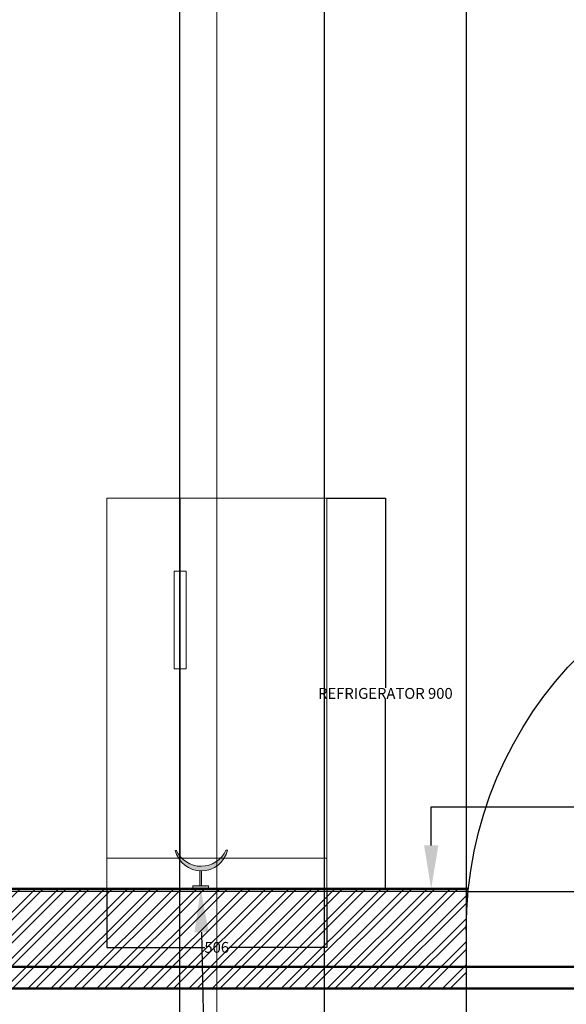
# Model space of a CAD drawing. Units: millimetres. Extents: x 1944 to 29915, y -10550 to 5909.
# Tile 5 of 24: x 7967 to 9226, y -5 to 2263. Entities that reach past the tile are written whole.
import ezdxf
from ezdxf import colors
from ezdxf.entities.mleader import LeaderData, LeaderLine
from ezdxf.math import Vec2, Vec3

# ---------------------------------------------------------------- set-up
doc = ezdxf.new("R2010")
doc.units = ezdxf.units.MM
doc.header["$MEASUREMENT"] = 0
for name, color, linetype, lineweight in [('A-ANNO-DIMS', 2, 'Continuous', 18), ('A-ANNO-SYMB', 2, 'Continuous', 18), ('A-ANNO-TEXT', 7, 'Continuous', 25), ('A-DOOR', 4, 'Continuous', 25), ('A-FLOR-FIXT', 9, 'Continuous', 18), ('A-FURN', 8, 'Continuous', 18), ('A-WALL', 7, 'Continuous', 50), ('A-WALL-PATT', 8, 'Continuous', 18)]:
    doc.layers.add(name, color=color, linetype=linetype, lineweight=lineweight)
doc.styles.get("Standard").update_dxf_attribs({"font": 'arial.ttf'})
doc.dimstyles.get("Standard").update_dxf_attribs({"dimtxt": 25, "dimasz": 0.18, "dimexe": 0.18, "dimexo": 0.0625, "dimgap": 0.09, "dimtad": 0, "dimtih": 1, "dimtoh": 1, "dimdec": 0, "dimzin": 0, "dimdsep": 46, "dimtxsty": 'Standard', "dimcen": 0.09, "dimadec": 0, "dimazin": 0, "dimtfac": 1, "dimtdec": 0, "dimtofl": 0, "dimtmove": 0, "dimatfit": 3, "dimfxl": 1, "dimtolj": 1, "dimtzin": 0, "dimarcsym": 0})

# ---------------------------------------------------------------- blocks, each defined once
blk = doc.blocks.new('*U2')
for p, q in [((0, 0), (0, -6)), ((40, 0), (40, -6))]:
    blk.add_line(p, q)
blk.add_lwpolyline([(0, 0), (0, 40), (1.75, 40), (1.75, 0)], close=True)
blk.add_arc((0, 0), 40, 0, 90)
blk = doc.blocks.new('Refrigerator-2 door - 36 in front')
for p, q in [((12, 5), (12, 64)), ((0, 5), (36, 5))]:
    blk.add_line(p, q)
for points in [[(0, 0), (0, 64), (36, 64), (36, 0)], [(11, 36), (11, 52), (13, 52), (13, 36)]]:
    blk.add_lwpolyline(points, close=True)
blk = doc.blocks.new('COAT-HOOK')
blk.add_line((47.6, 3.3), (47.6, 0))
for centre, radius, start, end in [((61.9, 60.2), 61.9, 103.3534, 256.6466), ((73.3, 60.6), 62.7, 114.1736, 245.8264)]:
    blk.add_arc(centre, radius, start, end)
blk = doc.blocks.new('*D40')
at = {"layer": 'A-ANNO-DIMS', "color": 0, "lineweight": -2, "transparency": 16777216}
for p, q in [((8674.1, 1160.8), (8809.2, 1160.8)), ((8809.1, 1160.7), (8809.1, 723.9)), ((8809.1, 261), (8809.1, 697.8)), ((8674.1, 260.8), (8809.2, 260.8))]:
    blk.add_line(p, q, dxfattribs=at)
at = {"layer": 'A-ANNO-DIMS', "color": 0, "transparency": 16777216}
for points in [[(8809, 1160.7), (8809.1, 1160.7), (8809.1, 1160.8)], [(8809, 261), (8809.1, 261), (8809.1, 260.8)]]:
    blk.add_solid(points, dxfattribs=at)
at = {"layer": 'Defpoints', "color": 0, "transparency": 16777216}
for p in [(8674.1, 1160.8), (8809.1, 1160.8), (8674.1, 260.8)]:
    blk.add_point(p, dxfattribs=at)
at = {"layer": 'A-ANNO-DIMS', "color": 0, "transparency": 16777216, "insert": (8809.1, 710.8), "char_height": 25, "attachment_point": 5}
blk.add_mtext('\\A1;REFRIGERATOR 900', dxfattribs=at)
blk = doc.blocks.new('*D41')
at = {"layer": 'A-ANNO-DIMS', "color": 0, "lineweight": -2, "transparency": 16777216}
for p, q in [((8167.8, 260.8), (8167.8, 125.7)), ((8674.1, 260.8), (8674.1, 125.7)), ((8168, 125.8), (8393.2, 125.8)), ((8673.9, 125.8), (8448.6, 125.8))]:
    blk.add_line(p, q, dxfattribs=at)
at = {"layer": 'A-ANNO-DIMS', "color": 0, "transparency": 16777216}
for points in [[(8168, 125.9), (8168, 125.8), (8167.8, 125.8)], [(8673.9, 125.9), (8673.9, 125.8), (8674.1, 125.8)]]:
    blk.add_solid(points, dxfattribs=at)
at = {"layer": 'Defpoints', "color": 0, "transparency": 16777216}
for p in [(8167.8, 260.8), (8674.1, 260.8), (8674.1, 125.8)]:
    blk.add_point(p, dxfattribs=at)
at = {"layer": 'A-ANNO-DIMS', "color": 0, "transparency": 16777216, "insert": (8420.9, 125.8), "char_height": 25, "attachment_point": 5}
blk.add_mtext('\\A1;506', dxfattribs=at)
blk = doc.blocks.new('*D49')
at = {"layer": 'A-ANNO-DIMS', "color": 0, "lineweight": -2, "transparency": 16777216}
for p, q in [((8335.5, 4760.8), (8335.5, -697.2)), ((6945.9, 4530.8), (6945.9, -697.2)), ((6946.1, -697), (7589.8, -697)), ((8335.3, -697), (7691.6, -697))]:
    blk.add_line(p, q, dxfattribs=at)
at = {"layer": 'A-ANNO-DIMS', "color": 0, "transparency": 16777216}
for points in [[(6946.1, -697), (6946.1, -697.1), (6945.9, -697)], [(8335.3, -697), (8335.3, -697.1), (8335.5, -697)]]:
    blk.add_solid(points, dxfattribs=at)
at = {"layer": 'Defpoints', "color": 0, "transparency": 16777216}
for p in [(8335.5, 4760.8), (6945.9, 4530.8), (8335.5, -697)]:
    blk.add_point(p, dxfattribs=at)
at = {"layer": 'A-ANNO-DIMS', "color": 0, "transparency": 16777216, "insert": (7640.7, -697), "char_height": 25, "attachment_point": 5}
blk.add_mtext('\\A1;1389.5', dxfattribs=at)
blk = doc.blocks.new('*D50')
at = {"layer": 'A-ANNO-DIMS', "color": 0, "lineweight": -2, "transparency": 16777216}
for p, q in [((8995.2, 30.8), (8995.2, -697.2)), ((9895.2, 30.8), (9895.2, -697.2)), ((8995.4, -697), (9417.6, -697)), ((9895, -697), (9472.9, -697))]:
    blk.add_line(p, q, dxfattribs=at)
at = {"layer": 'A-ANNO-DIMS', "color": 0, "transparency": 16777216}
for points in [[(8995.4, -697), (8995.4, -697.1), (8995.2, -697)], [(9895, -697), (9895, -697.1), (9895.2, -697)]]:
    blk.add_solid(points, dxfattribs=at)
at = {"layer": 'Defpoints', "color": 0, "transparency": 16777216}
for p in [(8995.2, 30.8), (9895.2, 30.8), (9895.2, -697)]:
    blk.add_point(p, dxfattribs=at)
at = {"layer": 'A-ANNO-DIMS', "color": 0, "transparency": 16777216, "insert": (9445.2, -697), "char_height": 25, "attachment_point": 5}
blk.add_mtext('\\A1;900', dxfattribs=at)
blk = doc.blocks.new('*D53')
at = {"layer": 'A-ANNO-DIMS', "color": 0, "lineweight": -2, "transparency": 16777216}
for p, q in [((6945.94205, 490.774608), (6945.94205, -697.212556)), ((9895.94205, 490.774608), (9895.94205, -697.212556)), ((6946.12205, -697.032556), (8383.35205, -697.032556)), ((9895.76205, -697.032556), (8458.53205, -697.032556))]:
    blk.add_line(p, q, dxfattribs=at)
at = {"layer": 'A-ANNO-DIMS', "color": 0, "transparency": 16777216}
for points in [[(6946.12205, -697.002556), (6946.12205, -697.062556), (6945.94205, -697.032556)], [(9895.76205, -697.002556), (9895.76205, -697.062556), (9895.94205, -697.032556)]]:
    blk.add_solid(points, dxfattribs=at)
at = {"layer": 'Defpoints', "color": 0, "transparency": 16777216}
for p in [(6945.94205, 490.837108), (9895.94205, 490.837108), (9895.94205, -697.032556)]:
    blk.add_point(p, dxfattribs=at)
at = {"layer": 'A-ANNO-DIMS', "color": 0, "transparency": 16777216, "insert": (8420.94205, -697.032556), "char_height": 25, "attachment_point": 5}
blk.add_mtext('\\A1;2950', dxfattribs=at)
blk = doc.blocks.new('*D56')
at = {"layer": 'A-ANNO-DIMS', "color": 0, "lineweight": -2, "transparency": 16777216}
for p, q in [((8999.7, 254.8), (11007.7, 254.8)), ((11007.5, 254.6), (11007.5, 155.7)), ((11007.5, 31), (11007.5, 130)), ((8995.3, 30.8), (11007.7, 30.8))]:
    blk.add_line(p, q, dxfattribs=at)
at = {"layer": 'A-ANNO-DIMS', "color": 0, "transparency": 16777216}
for points in [[(11007.5, 254.6), (11007.5, 254.6), (11007.5, 254.8)], [(11007.5, 31), (11007.5, 31), (11007.5, 30.8)]]:
    blk.add_solid(points, dxfattribs=at)
at = {"layer": 'Defpoints', "color": 0, "transparency": 16777216}
for p in [(8999.6, 254.8), (8995.2, 30.8), (11007.5, 30.8)]:
    blk.add_point(p, dxfattribs=at)
at = {"layer": 'A-ANNO-DIMS', "color": 0, "transparency": 16777216, "insert": (11007.5, 142.8), "char_height": 25, "attachment_point": 5}
blk.add_mtext('\\A1;223.95', dxfattribs=at)
blk = doc.blocks.new('*D57')
at = {"layer": 'A-ANNO-DIMS', "color": 0, "lineweight": -2, "transparency": 16777216}
for p, q in [((8995.2, 4760.8), (5803.8, 4760.8)), ((5804, 4760.7), (5804, 2520.7)), ((5804, 255), (5804, 2495)), ((8999.6, 254.8), (5803.8, 254.8))]:
    blk.add_line(p, q, dxfattribs=at)
at = {"layer": 'A-ANNO-DIMS', "color": 0, "transparency": 16777216}
for points in [[(5804, 4760.7), (5804, 4760.7), (5804, 4760.8)], [(5804, 255), (5804, 255), (5804, 254.8)]]:
    blk.add_solid(points, dxfattribs=at)
at = {"layer": 'Defpoints', "color": 0, "transparency": 16777216}
for p in [(8995.2, 4760.8), (5804, 254.8), (8999.6, 254.8)]:
    blk.add_point(p, dxfattribs=at)
at = {"layer": 'A-ANNO-DIMS', "color": 0, "transparency": 16777216, "insert": (5804, 2507.8), "char_height": 25, "attachment_point": 5}
blk.add_mtext('\\A1;4506', dxfattribs=at)
blk = doc.blocks.new('*D59')
at = {"layer": 'A-ANNO-DIMS', "color": 0, "lineweight": -2, "transparency": 16777216}
for p, q in [((8668, 4019.6), (8668, -697.2)), ((8995.2, 3870.8), (8995.2, -697.2)), ((8668.2, -697), (8789.5, -697)), ((8995, -697), (8873.8, -697))]:
    blk.add_line(p, q, dxfattribs=at)
at = {"layer": 'A-ANNO-DIMS', "color": 0, "transparency": 16777216}
for points in [[(8668.2, -697), (8668.2, -697.1), (8668, -697)], [(8995, -697), (8995, -697.1), (8995.2, -697)]]:
    blk.add_solid(points, dxfattribs=at)
at = {"layer": 'Defpoints', "color": 0, "transparency": 16777216}
for p in [(8668, 4019.6), (8995.2, 3870.8), (8995.2, -697)]:
    blk.add_point(p, dxfattribs=at)
at = {"layer": 'A-ANNO-DIMS', "color": 0, "transparency": 16777216, "insert": (8831.6, -697), "char_height": 25, "attachment_point": 5}
blk.add_mtext('\\A1;327.2', dxfattribs=at)

msp = doc.modelspace()

# ---------------------------------------------------------------- hatches: boundary and pattern name
at = {"layer": 'A-ANNO-SYMB'}
h = msp.add_hatch(color=256, dxfattribs=at)
h.dxf.hatch_style = 1
h.paths.add_polyline_path([(8445.574, 349.638), (8442.267, 349.638, -0.64725624), (8327.774, 349.638), (8325.088, 349.638, 0.79041326)])
h = msp.add_hatch(color=256, dxfattribs=at)
h.dxf.hatch_style = 1
h.paths.add_polyline_path([(8382.09, 267.383), (8386.174, 267.383), (8386.174, 302.026, -0.01650068), (8382.09, 302.106)])
h = msp.add_hatch(color=256, dxfattribs=at)
h.dxf.hatch_style = 1
h.paths.add_polyline_path([(8402.167, 260.837), (8402.167, 267.383), (8365.937, 267.383), (8365.937, 260.837)])
at = {"layer": 'A-WALL-PATT'}
h = msp.add_hatch(dxfattribs=at)
h.set_pattern_fill('ANSI32', color=256, scale=100)
h.paths.add_polyline_path([(6945.942, 260.837), (6945.942, 30.837), (8995.217, 30.837), (8995.217, 165.837, -0.0264443), (9000.245, 260.837)])

# ---------------------------------------------------------------- linework, layer by layer
at = {"layer": 'A-ANNO-SYMB'}
msp.add_line((8420.942, -176.269), (8420.942, 5412.489), dxfattribs=at)
at = {"layer": 'A-FLOR-FIXT'}
for p, q in [((8382.09, 302.089), (8382.09, 267.383)), ((8386.174, 302.089), (8386.174, 267.383))]:
    msp.add_line(p, q, dxfattribs=at)
for points in [[(8995.217, 30.837), (6715.942, 30.837), (6715.942, 4990.837), (8315.477, 4990.837)], [(9000.245, 260.837), (6945.942, 260.837), (6945.942, 4760.837), (8315.477, 4760.837)]]:
    msp.add_lwpolyline(points, dxfattribs=at)
msp.add_lwpolyline([(8402.167, 260.837), (8365.937, 260.837), (8365.937, 267.383), (8402.167, 267.383)], close=True, dxfattribs=at)
at = {"layer": 'A-WALL'}
for p, q in [((6945.942, 260.837), (9000.245, 260.837)), ((10125.942, 81.017), (6715.942, 81.017)), ((10125.942, 30.837), (6715.942, 30.837)), ((8995.217, 30.837), (9895.942, 30.837))]:
    msp.add_line(p, q, dxfattribs=at)

# ---------------------------------------------------------------- block references
at = {"layer": 'A-DOOR', "xscale": -22.5, "yscale": 22.5, "zscale": 22.5}
msp.add_blockref('*U2', (9895.217, 165.837), dxfattribs=at)
at = {"layer": 'A-FLOR-FIXT', "xscale": 14.0625, "yscale": 14.0625, "zscale": 14.0625}
msp.add_blockref('Refrigerator-2 door - 36 in front', (8167.817, 260.837), dxfattribs=at)
at = {"layer": 'A-FURN', "rotation": 90.14209801514701}
msp.add_blockref('COAT-HOOK', (8445.704, 302.134), dxfattribs=at)

# ---------------------------------------------------------------- dimensions: what is measured, and where the dimension line sits
at = {"layer": 'A-ANNO-DIMS'}
for base, p1, p2, override, picture, middle in [((5803.984, 254.791), (8995.217, 4760.837), (8999.621, 254.791), {"dimdec": 0, "dimlfac": 1, "dimrnd": 0, "dimzin": 0, "dimdsep": 46, "dimlunit": 2}, '*D57', (5803.984, 2507.814)), ((11007.504, 30.837), (8999.621, 254.791), (8995.217, 30.837), {"dimdec": 2, "dimlfac": 1, "dimrnd": 0, "dimzin": 0, "dimdsep": 46, "dimlunit": 2}, '*D56', (11007.504, 142.814))]:
    dim = msp.add_linear_dim(base=base, p1=p1, p2=p2, angle=90, dimstyle='Standard', override=override, dxfattribs=at)
    dim.commit()
    dim.dimension.update_dxf_attribs({"geometry": picture, "text_midpoint": middle})
for base, p1, p2, override, picture, middle in [((8335.477, -697.033), (6945.942, 4530.837), (8335.477, 4760.837), {"dimdec": 1, "dimlfac": 1, "dimrnd": 0, "dimzin": 0, "dimdsep": 46, "dimlunit": 2}, '*D49', (7640.71, -697.033)), ((8995.217, -697.033), (8668.038, 4019.643), (8995.217, 3870.837), {"dimdec": 1, "dimlfac": 1, "dimrnd": 0, "dimzin": 0, "dimdsep": 46, "dimlunit": 2}, '*D59', (8831.628, -697.033)), ((9895.942, -697.033), (6945.942, 490.837), (9895.942, 490.837), {"dimdec": 0, "dimlfac": 1, "dimrnd": 0, "dimzin": 0, "dimdsep": 46, "dimlunit": 2}, '*D53', (8420.942, -697.033)), ((8674.067, 125.837), (8167.817, 260.837), (8674.067, 260.837), {"dimdec": 0, "dimrnd": 0, "dimzin": 0, "dimlunit": 2}, '*D41', (8420.942, 125.837)), ((9895.217, -697.033), (8995.217, 30.837), (9895.217, 30.837), {"dimdec": 0, "dimlfac": 1, "dimrnd": 0, "dimzin": 0, "dimdsep": 46, "dimlunit": 2}, '*D50', (9445.217, -697.033))]:
    dim = msp.add_linear_dim(base=base, p1=p1, p2=p2, dimstyle='Standard', override=override, dxfattribs=at)
    dim.commit()
    dim.dimension.update_dxf_attribs({"geometry": picture, "text_midpoint": middle})
dim = msp.add_linear_dim(base=(8809.067, 1160.837), p1=(8674.067, 260.837), p2=(8674.067, 1160.837), angle=90, text='REFRIGERATOR <>', dimstyle='Standard', override={"dimdec": 0, "dimrnd": 0, "dimzin": 0, "dimlunit": 2}, dxfattribs=at)
dim.commit()
dim.dimension.update_dxf_attribs({"geometry": '*D40', "text_midpoint": (8809.067, 710.837)})

# ---------------------------------------------------------------- leaders
at = {"layer": 'A-ANNO-TEXT'}
ml = msp.add_multileader_mtext('Standard', dxfattribs=at)
ml.set_content('SWITCH BOARD', color=256)
ml.set_leader_properties()
ml.build(insert=Vec2(0, 0))
ml.multileader.update_dxf_attribs({"dogleg_length": 568.936, "arrow_head_size": 100})
ctx = ml.context
ctx.base_point, ctx.char_height, ctx.arrow_head_size, ctx.landing_gap_size, ctx.plane_origin = Vec3(11122.176, 449.474), 100, 100, 0.09, Vec3(10553.24, 449.474)
ctx.text_align_type = 2
notes = []
notes.append((ctx, [(0, (1, 1, 0), (10553.24, 449.474), (1, 0), 568.936, [(0, [(8914.665, 260.837), (8914.665, 449.474)], 0, [])])]))
ctx.mtext.insert, ctx.mtext.alignment, ctx.mtext.flow_direction = Vec3(12195.117, 500.327), 3, 5
ml = msp.add_multileader_mtext('Standard', dxfattribs=at)
ml.set_content('15 AMP POWER POINT \\PFOR MIXER', color=256)
ml.set_leader_properties()
ml.build(insert=Vec2(0, 0))
ml.multileader.update_dxf_attribs({"dogleg_length": 568.936, "arrow_head_size": 100})
ctx = ml.context
ctx.base_point, ctx.char_height, ctx.arrow_head_size, ctx.landing_gap_size, ctx.plane_origin = Vec3(4878.252, -422.117), 100, 100, 0.09, Vec3(6870.097, -798.764)
ctx.text_align_type = 2
notes.append((ctx, [(0, (1, 1, 0), (6958.555, -422.117), (-1, 0), 568.936, [(0, [(8384.052, 260.837), (8397.606, -446.246)], 0, [])])]))
ctx.mtext.insert, ctx.mtext.alignment, ctx.mtext.flow_direction = Vec3(6389.529, -371.264), 3, 5
for ctx, leaders in notes:
    for number, flags, end, landing, length, lines in leaders:
        leader = LeaderData()
        leader.index, (leader.has_last_leader_line, leader.has_dogleg_vector, leader.attachment_direction) = number, flags
        leader.last_leader_point, leader.dogleg_vector, leader.dogleg_length = Vec3(end), Vec3(landing), length
        for number, points, colour, breaks in lines:
            line = LeaderLine()
            line.index, line.vertices, line.color, line.breaks = number, Vec3.list(points), colors.encode_raw_color(colour), breaks
            leader.lines.append(line)
        ctx.leaders.append(leader)

doc.saveas('drawing.dxf')
